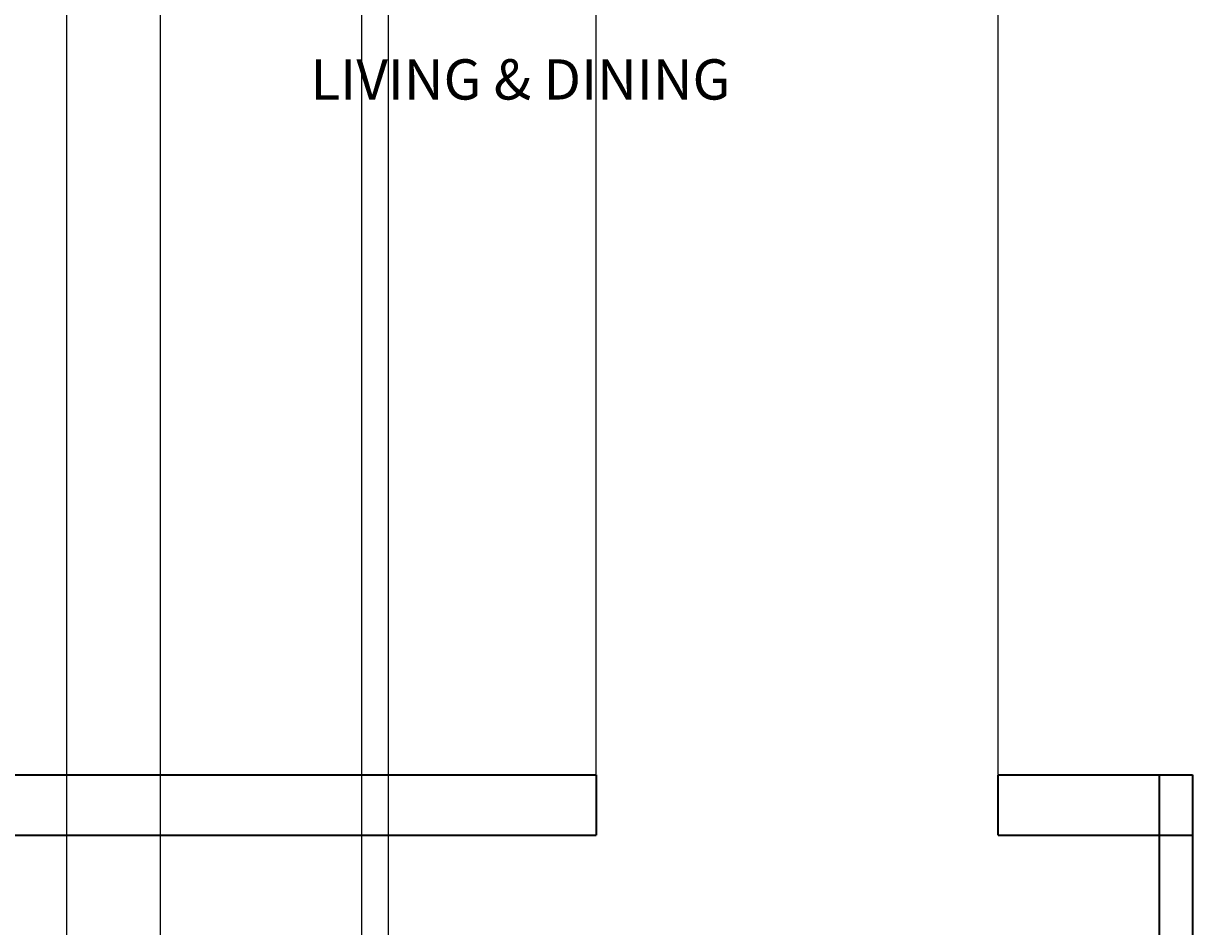
# Model space of a CAD drawing. Units: inches. Extents: x 450 to 1026, y 542 to 1190.
# Tile 6 of 11: x 632 to 807, y 804 to 939. Entities that reach past the tile are written whole.
import ezdxf

# ---------------------------------------------------------------- set-up
doc = ezdxf.new("R2010")
doc.units = ezdxf.units.IN
doc.header["$MEASUREMENT"] = 0
for name, color, linetype, lineweight in [('A-ANNO-DIMS', 2, 'Continuous', 18), ('A-AREA-IDEN', 7, 'Continuous', 18), ('A-WALL', 7, 'Continuous', 35)]:
    doc.layers.add(name, color=color, linetype=linetype, lineweight=lineweight)
doc.styles.get("Standard").update_dxf_attribs({"font": 'arial.ttf'})
doc.dimstyles.get("Standard").update_dxf_attribs({"dimtxt": 0.18, "dimasz": 0.18, "dimexe": 0.18, "dimexo": 0.0625, "dimgap": 0.09, "dimtad": 0, "dimtih": 1, "dimtoh": 1, "dimdec": 4, "dimzin": 0, "dimdsep": 46, "dimtxsty": 'Standard', "dimcen": 0.09, "dimadec": 0, "dimazin": 0, "dimtfac": 1, "dimtdec": 4, "dimtofl": 0, "dimtmove": 0, "dimatfit": 3, "dimfxl": 1, "dimtolj": 1, "dimtzin": 0, "dimarcsym": 0})

# ---------------------------------------------------------------- blocks, each defined once
blk = doc.blocks.new('*D53')
at = {"layer": 'A-ANNO-DIMS', "color": 0, "lineweight": -2, "transparency": 16777216}
for p, q in [((479.59, 817.94), (449.87, 817.94)), ((450.05, 817.76), (450.05, 706.62)), ((450.05, 595.12), (450.05, 706.26)), ((797.59, 594.94), (449.87, 594.94))]:
    blk.add_line(p, q, dxfattribs=at)
at = {"layer": 'A-ANNO-DIMS', "color": 0, "transparency": 16777216}
for points in [[(450.02, 817.76), (450.08, 817.76), (450.05, 817.94)], [(450.02, 595.12), (450.08, 595.12), (450.05, 594.94)]]:
    blk.add_solid(points, dxfattribs=at)
at = {"layer": 'Defpoints', "color": 0, "transparency": 16777216}
for p in [(479.65, 817.94), (450.05, 594.94), (797.65, 594.94)]:
    blk.add_point(p, dxfattribs=at)
at = {"layer": 'A-ANNO-DIMS', "color": 0, "transparency": 16777216, "insert": (450.05, 706.44), "char_height": 0.18, "attachment_point": 5}
blk.add_mtext('\\A1;223', dxfattribs=at)
blk = doc.blocks.new('*D57')
at = {"layer": 'A-ANNO-DIMS', "color": 0, "lineweight": -2, "transparency": 16777216}
for p, q in [((638.65, 970.88), (638.65, 542.16)), ((686.65, 970.88), (686.65, 542.16)), ((638.83, 542.34), (662.43, 542.34)), ((686.47, 542.34), (662.87, 542.34))]:
    blk.add_line(p, q, dxfattribs=at)
at = {"layer": 'A-ANNO-DIMS', "color": 0, "transparency": 16777216}
for points in [[(638.83, 542.37), (638.83, 542.31), (638.65, 542.34)], [(686.47, 542.37), (686.47, 542.31), (686.65, 542.34)]]:
    blk.add_solid(points, dxfattribs=at)
at = {"layer": 'Defpoints', "color": 0, "transparency": 16777216}
for p in [(638.65, 970.94), (686.65, 970.94), (686.65, 542.34)]:
    blk.add_point(p, dxfattribs=at)
at = {"layer": 'A-ANNO-DIMS', "color": 0, "transparency": 16777216, "insert": (662.65, 542.34), "char_height": 0.18, "attachment_point": 5}
blk.add_mtext('\\A1;48', dxfattribs=at)
blk = doc.blocks.new('*D60')
at = {"layer": 'A-ANNO-DIMS', "color": 0, "lineweight": -2, "transparency": 16777216}
for p, q in [((717.65, 827.01), (717.65, 1189.72)), ((777.65, 827.01), (777.65, 1189.72)), ((717.83, 1189.54), (747.43, 1189.54)), ((777.47, 1189.54), (747.87, 1189.54))]:
    blk.add_line(p, q, dxfattribs=at)
at = {"layer": 'A-ANNO-DIMS', "color": 0, "transparency": 16777216}
for points in [[(717.83, 1189.57), (717.83, 1189.51), (717.65, 1189.54)], [(777.47, 1189.57), (777.47, 1189.51), (777.65, 1189.54)]]:
    blk.add_solid(points, dxfattribs=at)
at = {"layer": 'Defpoints', "color": 0, "transparency": 16777216}
for p in [(777.65, 1189.54), (717.65, 826.94), (777.65, 826.94)]:
    blk.add_point(p, dxfattribs=at)
at = {"layer": 'A-ANNO-DIMS', "color": 0, "transparency": 16777216, "insert": (747.65, 1189.54), "char_height": 0.18, "attachment_point": 5}
blk.add_mtext('\\A1;60', dxfattribs=at)
blk = doc.blocks.new('*D66')
at = {"layer": 'A-ANNO-DIMS', "color": 0, "lineweight": -2, "transparency": 16777216}
for p, q in [((652.65, 1018.88), (652.65, 542.16)), ((682.65, 1018.88), (682.65, 542.16)), ((652.83, 542.34), (667.43, 542.34)), ((682.47, 542.34), (667.87, 542.34))]:
    blk.add_line(p, q, dxfattribs=at)
at = {"layer": 'A-ANNO-DIMS', "color": 0, "transparency": 16777216}
for points in [[(652.83, 542.37), (652.83, 542.31), (652.65, 542.34)], [(682.47, 542.37), (682.47, 542.31), (682.65, 542.34)]]:
    blk.add_solid(points, dxfattribs=at)
at = {"layer": 'Defpoints', "color": 0, "transparency": 16777216}
for p in [(652.65, 1018.94), (682.65, 1018.94), (682.65, 542.34)]:
    blk.add_point(p, dxfattribs=at)
at = {"layer": 'A-ANNO-DIMS', "color": 0, "transparency": 16777216, "insert": (667.65, 542.34), "char_height": 0.18, "attachment_point": 5}
blk.add_mtext('\\A1;30', dxfattribs=at)

msp = doc.modelspace()

# ---------------------------------------------------------------- linework, layer by layer
at = {"layer": 'A-WALL'}
for p, q in [((536.6513, 826.9426), (717.6513, 826.9426)), ((717.6513, 826.9426), (717.6513, 817.9426)), ((777.6513, 817.9426), (777.6513, 826.9426)), ((777.6513, 826.9426), (806.6513, 826.9426)), ((801.6513, 826.9426), (801.6513, 673.9426)), ((806.6513, 826.9426), (806.6513, 603.9426)), ((479.6513, 817.9426), (717.6513, 817.9426)), ((777.6513, 817.9426), (806.6513, 817.9426))]:
    msp.add_line(p, q, dxfattribs=at)

# ---------------------------------------------------------------- texts
at = {"layer": 'A-AREA-IDEN'}
msp.add_text('LIVING & DINING', height=6, dxfattribs=at).set_placement((675.0435, 927.6384))

# ---------------------------------------------------------------- dimensions: what is measured, and where the dimension line sits
at = {"layer": 'A-ANNO-DIMS'}
for base, p1, p2, picture, middle in [((777.6513, 1189.5426), (717.6513, 826.9426), (777.6513, 826.9426), '*D60', (747.6513, 1189.5426)), ((682.6513, 542.3426), (652.6513, 1018.9426), (682.6513, 1018.9426), '*D66', (667.6513, 542.3426)), ((686.6513, 542.3426), (638.6513, 970.9426), (686.6513, 970.9426), '*D57', (662.6513, 542.3426))]:
    dim = msp.add_linear_dim(base=base, p1=p1, p2=p2, dimstyle='Standard', override={"dimdec": 0, "dimlfac": 1, "dimrnd": 0, "dimzin": 0, "dimdsep": 46, "dimlunit": 2}, dxfattribs=at)
    dim.commit()
    dim.dimension.update_dxf_attribs({"geometry": picture, "text_midpoint": middle})
dim = msp.add_linear_dim(base=(450.0513, 594.9426), p1=(479.6513, 817.9426), p2=(797.6513, 594.9426), angle=90, dimstyle='Standard', override={"dimdec": 0, "dimlfac": 1, "dimrnd": 0, "dimzin": 0, "dimdsep": 46, "dimlunit": 2}, dxfattribs=at)
dim.commit()
dim.dimension.update_dxf_attribs({"geometry": '*D53', "text_midpoint": (450.0513, 706.4426)})

doc.saveas('drawing.dxf')
